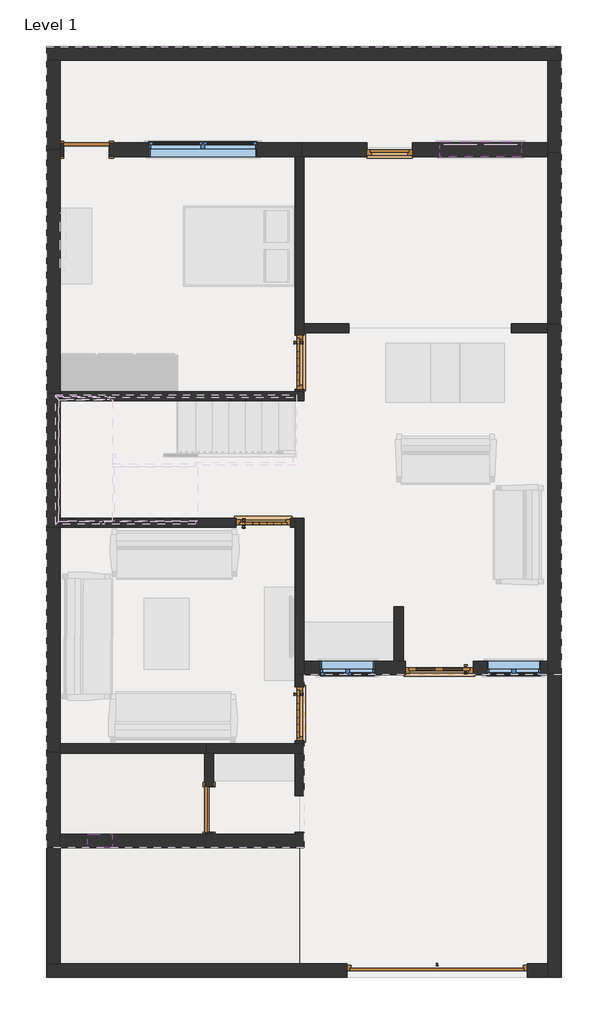
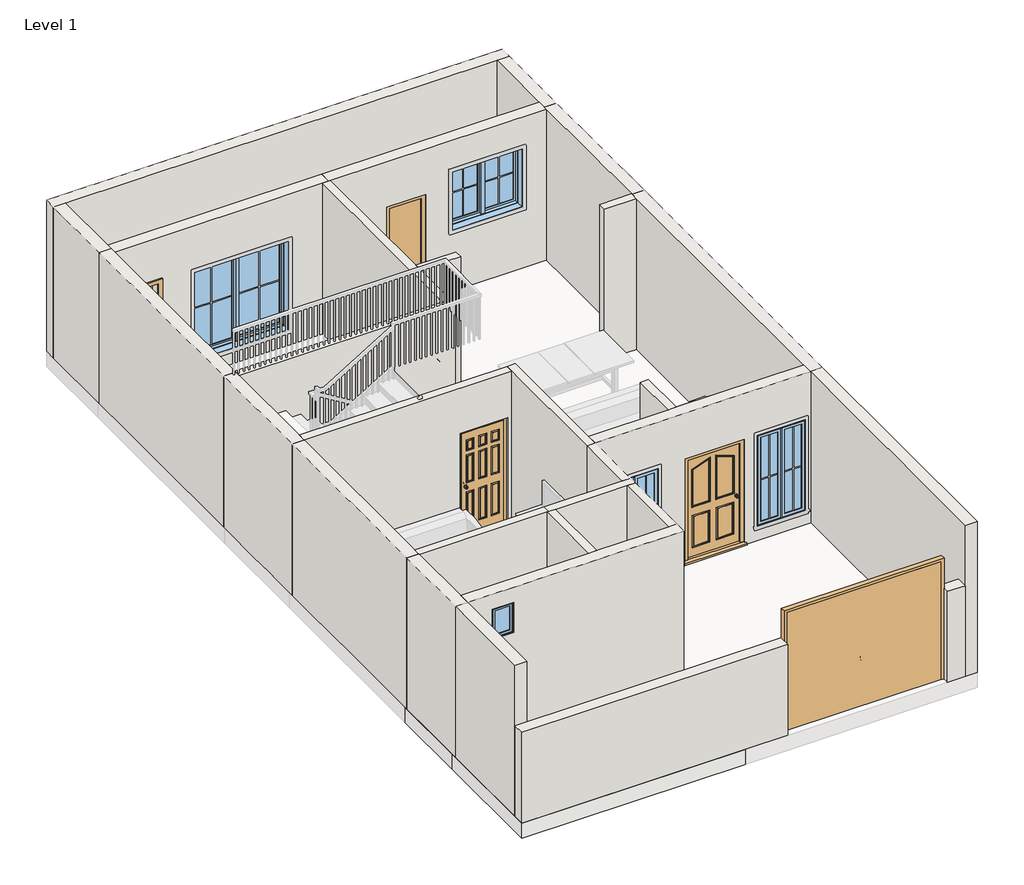
# One storey, part 1 of 3: 28 walls, 8 doors, 5 windows, 2 slabs.
# Revit data of these elements (continued)
# Materials (continued)
#   "Sash": class "Wood", colour RGB 224 178 126, transparency 0, Cost = 0
#   "Wood - Stained": class "Wood", colour RGB 224 178 126, transparency 0, Cost = 0
#   "Clad - White": class "Wood", colour RGB 242 242 238, transparency 0, Cost = 0
#   "Default Floor": colour RGB 128 128 128, transparency 0, Cost = 0
#   "Tile, Porcelain, 4in": class "Generic", colour RGB 89 87 158, transparency 0, Description = "Porcelain tile, 4\", white", Cost = 0
#   "FRONT WALL": class "Generic", colour RGB 120 120 120, transparency 0, Cost = 0
#   "Grass": class "Generic", colour RGB 104 137 66, transparency 0, Description = "Physical material.", Cost = 0
#   "Brick, Common": class "Masonry", colour RGB 170 98 104, transparency 0, Description = "Common brick", Cost = 0
#   "Default Wall": colour RGB 128 128 128, transparency 0, Cost = 0
#   "WALL 2": class "Generic", colour RGB 120 120 120, transparency 0, Cost = 0
#   "WALL 8": class "Generic", colour RGB 120 120 120, transparency 0, Cost = 0
#   "Copper": class "Metal", colour RGB 0 0 0, transparency 0, Description = "Copper, matte finish", Cost = 0
#   "HALL WALL 2": class "Generic", colour RGB 120 120 120, transparency 0, Cost = 0
#   "WALL HALL": class "Generic", colour RGB 120 120 120, transparency 0, Cost = 0
#   "PARKING FLOOR": class "Generic", colour RGB 120 120 120, transparency 0, Cost = 0
#   "BATH WALL1": class "Generic", colour RGB 120 120 120, transparency 0, Cost = 0
#   "wall7": class "Generic", colour RGB 120 120 120, transparency 0, Cost = 0
